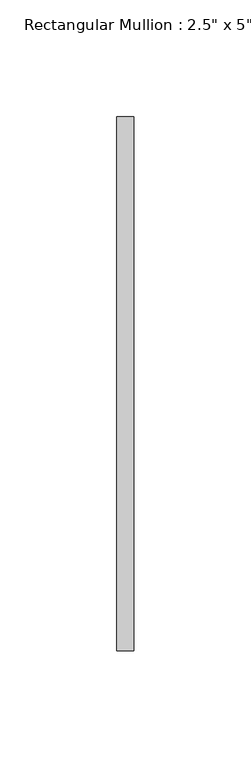
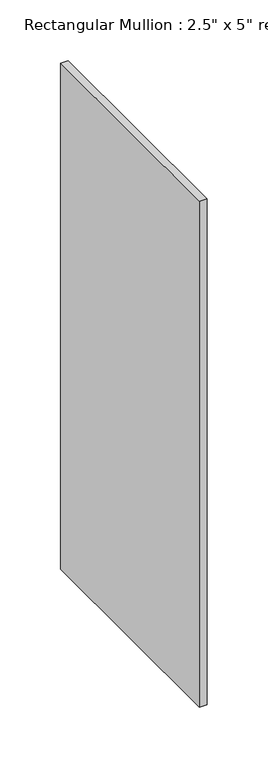
"""IFC4 building model written with IfcOpenShell, lengths in millimetres: member geometry."""

from ifc_helpers import new_model, si_unit, frame, origin, place, context, project, spatial, polyline, outline, extrude, source, transform, mapped, element, save


def member_0fd823d9(model_context):
    return source(origin(), model_context, "Body", "SweptSolid", [
        extrude(outline(polyline([(3.6195, 114.3), (3.6195, -114.3), (-3.6195, -114.3), (-3.6195, 114.3), (3.6195, 114.3)])), frame((0.0, 0.0, -508.0), z_axis=(0.0, 0.0, 1.0), x_axis=(1.0, 0.0, 0.0)), (0.0, 0.0, 1.0), 508.0),
    ])


if __name__ == "__main__":
    model = new_model("IFC4")
    model_context = context("Model", 3, world=origin())
    ifc_project = project(units=[si_unit("LENGTHUNIT", "METRE", prefix="MILLI")], contexts=[model_context])
    site = spatial("IfcSite", under=ifc_project)
    building = spatial("IfcBuilding", under=site)
    placement = place(None, origin())
    member_shape = member_0fd823d9(model_context)
    element("IfcMember", 1, ObjectType="Rectangular Mullion : 2.5\" x 5\" rectangular", at=placement, inside=building, context=model_context, shape_type="MappedRepresentation", body=[
        mapped(member_shape, transform((0.0, 0.0, 0.0), x_axis=(1.0, 0.0, 0.0), y_axis=(0.0, 1.0, 0.0), z_axis=(0.0, 0.0, 1.0))),
    ])
    save(model, "model.ifc")

# Revit data of these elements
# Type "Rectangular Mullion : 2.5\" x 5\" rectangular"
#   built-in parameter 1007304 = 0.75 (stored number, unit not read)
#   built-in parameter 1007301 = 0.011875 (stored number, unit not read)
#   built-in parameter 1007300 = 0.011875 (stored number, unit not read)
# Element 1 (IfcMember, "Rectangular Mullion : 2.5\" x 5\" rectangular")
#   Materials on its faces: "WINDOW GLASS MATERIAL"
# Materials
#   "WINDOW GLASS MATERIAL": class "Generic", colour RGB 120 120 120, transparency 0, Cost = 0
